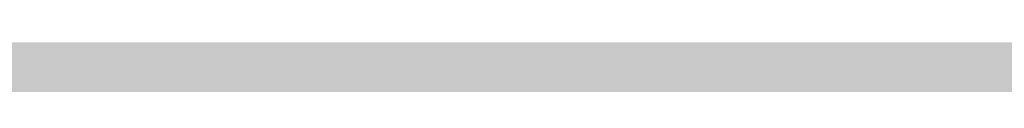
# Model space of a CAD drawing. Units: feet. Extents: x 3168 to 4724, y 827 to 1477.
# Tile 151 of 256: x 3301.1638 to 3301.19778, y 1099.01485 to 1099.01628. Entities that reach past the tile are written whole.
import ezdxf

# ---------------------------------------------------------------- set-up
doc = ezdxf.new("R2010")
doc.units = ezdxf.units.FT
doc.layers.add('A-ELEV', color=7, linetype='Continuous', lineweight=35)
doc.layers.add('A-ELEV-PATT', color=8, linetype='Continuous', lineweight=13)

msp = doc.modelspace()

# ---------------------------------------------------------------- hatches: boundary and pattern name
at = {"layer": 'A-ELEV-PATT'}
h = msp.add_hatch(color=256, dxfattribs=at)
h.dxf.hatch_style = 1
edge = h.paths.add_edge_path()
edge.add_ellipse((3552.905762, 979.220141), major_axis=(36.744924, 0), ratio=0.484848485, start_angle=0, end_angle=360)
edge = h.paths.add_edge_path()
edge.add_ellipse((3559.891637, 929.252282), major_axis=(36.744924, 0), ratio=0.484848485, start_angle=0, end_angle=360)
edge = h.paths.add_edge_path()
edge.add_line((3299.31681, 1198.606081), (3479.916714, 1198.606081))
edge.add_line((3479.916714, 1198.606081), (3479.916714, 1209.86857))
edge.add_spline(control_points=[(3479.916714, 1209.86857), (3464.301157, 1209.86857), (3448.685601, 1209.86857), (3410.949139, 1209.86857), (3388.828234, 1209.86857), (3355.646876, 1209.86857), (3344.586423, 1209.86857), (3327.995745, 1209.86857), (3322.465518, 1209.86857), (3314.170179, 1209.86857), (3311.405066, 1209.86857), (3307.257396, 1209.86857), (3305.874839, 1209.86857), (3303.801005, 1209.86857), (3303.109726, 1209.86857), (3302.072809, 1209.86857), (3301.72717, 1209.86857), (3301.208711, 1209.86857), (3301.035891, 1209.86857), (3300.776662, 1209.86857), (3300.690252, 1209.86857), (3300.560638, 1209.86857), (3300.517433, 1209.86857), (3300.452625, 1209.86857), (3300.431023, 1209.86857), (3300.398619, 1209.86857), (3300.387818, 1209.86857), (3300.366216, 1209.86857), (3300.345676, 1209.86857), (3300.345548, 1209.86857), (3300.345505, 1209.86857), (3300.343304, 1209.86857), (3300.341146, 1209.868571), (3300.337909, 1209.868571), (3300.33683, 1209.868572), (3300.333942, 1209.868573), (3300.332133, 1209.868574), (3300.325515, 1209.868577), (3300.320706, 1209.868581), (3300.310925, 1209.868592), (3300.305952, 1209.868598), (3300.290511, 1209.868623), (3300.280045, 1209.868646), (3300.232425, 1209.868777), (3300.195298, 1209.868954), (3299.951068, 1209.870608), (3299.744824, 1209.874326), (3299.436827, 1209.883257), (3299.334389, 1209.886792), (3299.181079, 1209.89292), (3299.130033, 1209.895099), (3298.652217, 1209.916801), (3298.22946, 1209.945718), (3297.601631, 1210.002367), (3297.393404, 1210.023464), (3297.082652, 1210.058309), (3296.979332, 1210.070458), (3296.292954, 1210.154861), (3295.718148, 1210.243356), (3294.868717, 1210.39885), (3294.5877, 1210.454478), (3294.169341, 1210.543349), (3294.030415, 1210.573878), (3291.707149, 1211.1012), (3289.65359, 1211.813435), (3285.776259, 1213.563988), (3283.95141, 1214.603478), (3280.512159, 1216.98008), (3278.897241, 1218.317592), (3276.379914, 1220.829489), (3275.416042, 1221.917738), (3274.039342, 1223.7077), (3273.581043, 1224.349535), (3273.143228, 1225.016316)], knot_values=[39.119033, 39.119033, 39.119033, 39.119033, 39.286353, 39.286353, 39.523379, 39.523379, 39.641892, 39.641892, 39.701148, 39.701148, 39.730777, 39.730777, 39.745591, 39.745591, 39.752998, 39.752998, 39.756701, 39.756701, 39.758553, 39.758553, 39.759479, 39.759479, 39.759942, 39.759942, 39.760173, 39.760173, 39.760289, 39.760289, 39.760405, 39.760405, 39.760463, 39.760463, 39.763389, 39.763389, 39.764851, 39.764851, 39.767304, 39.767304, 39.773825, 39.773825, 39.78057, 39.78057, 39.79477, 39.79477, 39.845194, 39.845194, 40.126715, 40.126715, 40.267476, 40.267476, 40.337856, 40.337856, 40.927023, 40.927023, 41.221606, 41.221606, 41.368898, 41.368898, 42.202622, 42.202622, 42.619485, 42.619485, 42.827916, 42.827916, 46.118323, 46.118323, 49.408731, 49.408731, 52.699139, 52.699139, 54.927489, 54.927489, 56.104228, 56.104228, 56.104228, 56.104228], weights=[1, 1, 1, 1, 1, 1, 1, 1, 1, 1, 1, 1, 1, 1, 1, 1, 1, 1, 1, 1, 1, 1, 1, 1, 1, 1, 1, 1, 1, 1, 1, 1, 1, 1, 1, 1, 1, 1, 1, 1, 1, 1, 1, 1, 1, 1, 1, 1, 1, 1, 1, 1, 1, 1, 1, 1, 1, 1, 1, 1, 1, 1, 1, 1, 1, 1, 1, 1, 1, 1, 1, 1, 1, 1], degree=3, periodic=0)
edge.add_line((3273.143228, 1225.016316), (3273.143228, 1099.016316))
edge.add_line((3273.143228, 1099.016316), (3299.31681, 1099.016316))
edge.add_line((3299.31681, 1099.016316), (3299.31681, 1198.606081))
edge = h.paths.add_edge_path()
edge.add_line((3304.758443, 1324.15806), (3479.916714, 1324.15806))
edge.add_line((3479.916714, 1324.15806), (3479.916714, 1335.714618))
edge.add_line((3479.916714, 1335.714618), (3269.161628, 1335.714618))
edge.add_spline(control_points=[(3269.161628, 1335.714618), (3264.024231, 1335.714618), (3258.364118, 1328.958189), (3259.264311, 1323.900274)], knot_values=[0, 0, 0, 0, 15.412191, 15.412191, 15.412191, 15.412191], degree=3, periodic=0)
edge.add_line((3259.264311, 1323.900274), (3265.516849, 1288.769135))
edge.add_line((3265.516849, 1288.769135), (3275.265103, 1261.545626))
edge.add_line((3275.265103, 1261.545626), (3304.758443, 1261.545626))
edge.add_line((3304.758443, 1261.545626), (3304.758443, 1324.15806))
h = msp.add_hatch(color=256, dxfattribs=at)
h.dxf.hatch_style = 1
h.paths.add_polyline_path([(3384.525247, 1099.016316), (3335.029168, 1099.016316), (3299.31681, 1099.016316), (3273.143228, 1099.016316), (3217.565364, 1099.016316), (3168.069285, 827.11626), (3335.029168, 827.11626)])

# ---------------------------------------------------------------- linework, layer by layer
at = {"layer": 'A-ELEV'}
msp.add_open_spline([(3808.5202, 1099.016316), (3808.5202, 1141.413235), (3808.5202, 1183.810154), (3808.5202, 1226.635324), (3808.5202, 1227.063576), (3808.5202, 1227.491828), (3811.491871, 1248.994673), (3814.463542, 1270.497518), (3817.46523, 1292.217564), (3817.495247, 1292.434764), (3817.525264, 1292.651964), (3817.572801, 1310.106748), (3817.620339, 1327.561532), (3817.667877, 1345.016316), (3817.667877, 1345.457962), (3817.667877, 1345.899608), (3817.667877, 1346.456047), (3817.667877, 1346.57084), (3817.667877, 1346.752887), (3817.667877, 1346.820142), (3817.667877, 1346.93487), (3817.667877, 1346.982345), (3817.667877, 1347.038587), (3817.667877, 1347.047356), (3817.667877, 1347.073661), (3817.667877, 1347.059303), (3817.667877, 1347.061545), (3817.667876, 1347.062667), (3817.667875, 1347.066031), (3817.667874, 1347.068274), (3817.66787, 1347.075001), (3817.667866, 1347.079486), (3817.667849, 1347.092937), (3817.667833, 1347.101902), (3817.667766, 1347.12879), (3817.667699, 1347.146705), (3817.667432, 1347.200421), (3817.667165, 1347.236192), (3817.6661, 1347.343385), (3817.665038, 1347.414686), (3817.660812, 1347.628095), (3817.656608, 1347.769708), (3817.63997, 1348.192487), (3817.623509, 1348.471586), (3817.559094, 1349.300067), (3817.496121, 1349.840588), (3817.255432, 1351.424156), (3817.026318, 1352.428785), (3816.306871, 1354.888914), (3815.743745, 1356.268727), (3814.463959, 1358.81921), (3813.746413, 1359.990968), (3812.195838, 1362.172343), (3811.362245, 1363.182124), (3809.588836, 1365.069009), (3808.648816, 1365.946105), (3806.654262, 1367.579616), (3805.599702, 1368.336154), (3803.352891, 1369.722327), (3802.160535, 1370.352386), (3799.600813, 1371.453586), (3798.232688, 1371.925481), (3795.280084, 1372.634624), (3793.693148, 1372.872068), (3791.869441, 1372.92648), (3791.740861, 1372.92922), (3791.353371, 1372.934101), (3791.092707, 1372.932901), (3790.304116, 1372.915068), (3789.769543, 1372.884195), (3789.20919, 1372.830236), (3789.190622, 1372.828424), (3789.134892, 1372.822912), (3789.097705, 1372.819137), (3789.048445, 1372.814008), (3789.0364, 1372.812743), (3789.000256, 1372.808918), (3788.976147, 1372.806325), (3788.949405, 1372.803404), (3788.946786, 1372.803118), (3788.942567, 1372.802655), (3788.940967, 1372.80248), (3788.938572, 1372.802217), (3788.937777, 1372.802129), (3788.935391, 1372.801867), (3788.867535, 1372.794402), (3788.756866, 1372.782228), (3788.701532, 1372.776141), (3788.53553, 1372.75788), (3788.424861, 1372.745707), (3788.092856, 1372.709185), (3787.871519, 1372.684837), (3787.207509, 1372.611793), (3786.764835, 1372.563097), (3785.436814, 1372.417009), (3784.551467, 1372.319617), (3781.895425, 1372.027442), (3780.12473, 1371.832658), (3774.812646, 1371.248307), (3771.271256, 1370.858739), (3760.647088, 1369.690037), (3753.56431, 1368.910902), (3732.315973, 1366.573498), (3718.150416, 1365.015228), (3694.006758, 1362.359326), (3684.028657, 1361.261694), (3674.050557, 1360.164062), (3664.600662, 1360.164062), (3655.150767, 1360.164062), (3626.801081, 1360.164062), (3607.901291, 1360.164062), (3551.20192, 1360.164062), (3513.40234, 1360.164062), (3467.725182, 1360.164062), (3459.847604, 1360.164062), (3436.214873, 1360.164062), (3420.459718, 1360.164062), (3373.194255, 1360.164062), (3341.683946, 1360.164062), (3302.848162, 1360.164062), (3295.522686, 1360.164062), (3286.038292, 1360.164062), (3283.879372, 1360.164062), (3277.402613, 1360.164062), (3273.084773, 1360.164062), (3267.732851, 1360.164062), (3266.698768, 1360.164062), (3263.59652, 1360.164062), (3261.528355, 1360.164062), (3259.236943, 1360.164062), (3259.013697, 1360.164062), (3258.343958, 1360.164062), (3257.897466, 1360.164062), (3257.430998, 1360.164062), (3257.411022, 1360.164062), (3257.370573, 1360.164062), (3257.37547, 1360.164062), (3257.374598, 1360.164062), (3257.373937, 1360.164062), (3257.371956, 1360.164062), (3257.370635, 1360.164061), (3257.366673, 1360.16406), (3257.364032, 1360.164059), (3257.356109, 1360.164053), (3257.350828, 1360.164047), (3257.334987, 1360.164023), (3257.32443, 1360.163998), (3257.292769, 1360.163899), (3257.271676, 1360.163799), (3257.208439, 1360.163398), (3257.166337, 1360.162995), (3257.040206, 1360.161388), (3256.956349, 1360.159783), (3256.705504, 1360.153393), (3256.53924, 1360.147036), (3256.04357, 1360.121916), (3255.717296, 1360.097102), (3254.752446, 1360.000481), (3254.127968, 1359.906513), (3252.180067, 1359.525332), (3250.941574, 1359.143991), (3248.670175, 1358.24329), (3247.635739, 1357.723834), (3245.732632, 1356.603471), (3244.863388, 1356.00206), (3243.253108, 1354.742865), (3242.511972, 1354.084731), (3240.751052, 1352.344781), (3239.800961, 1351.229574), (3238.087769, 1348.87244), (3237.324685, 1347.630355), (3235.98251, 1344.971632), (3235.402205, 1343.554907), (3234.591081, 1340.815458), (3234.310882, 1339.54355), (3233.97649, 1336.802561), (3233.922113, 1335.330877), (3234.148916, 1332.591269), (3234.349529, 1331.367201), (3234.719893, 1329.999367), (3234.752423, 1329.883362), (3234.853619, 1329.534797), (3234.925892, 1329.301685), (3235.024836, 1329.002552), (3235.046924, 1328.936928), (3235.077639, 1328.847239), (3235.085924, 1328.823198), (3235.110939, 1328.751064), (3235.127828, 1328.702962), (3235.147992, 1328.646242), (3235.151059, 1328.637632), (3235.156096, 1328.623526), (3235.158061, 1328.61803), (3235.160209, 1328.61203), (3235.165612, 1328.596943), (3235.180099, 1328.556486), (3235.190263, 1328.528101), (3235.220756, 1328.442946), (3235.241084, 1328.386176), (3235.302069, 1328.215865), (3235.342726, 1328.102325), (3235.464696, 1327.761704), (3235.54601, 1327.534623), (3235.78995, 1326.853381), (3235.952577, 1326.39922), (3236.440459, 1325.036736), (3236.765713, 1324.128414), (3237.741475, 1321.403446), (3238.391983, 1319.586801), (3240.343508, 1314.136866), (3241.644525, 1310.503576), (3245.547574, 1299.603706), (3248.149607, 1292.337126), (3255.955706, 1270.537385), (3261.159772, 1256.004225), (3267.387618, 1238.612001), (3268.411397, 1235.752937), (3269.510378, 1232.683864), (3269.585579, 1232.473854), (3269.706612, 1232.135851), (3269.752444, 1232.007857), (3269.827329, 1231.79873), (3269.856382, 1231.717595), (3269.906325, 1231.578122), (3269.927215, 1231.519782), (3269.972468, 1231.393406), (3269.996831, 1231.325368), (3270.026503, 1231.242506), (3270.031811, 1231.227681), (3270.040282, 1231.204024), (3270.039224, 1231.206979), (3270.039359, 1231.206601), (3270.039427, 1231.206412), (3270.03963, 1231.205846), (3270.039765, 1231.205468), (3270.040171, 1231.204335), (3270.040442, 1231.203579), (3270.041254, 1231.201313), (3270.041796, 1231.199802), (3270.04342, 1231.195269), (3270.044504, 1231.192248), (3270.047756, 1231.183185), (3270.049926, 1231.177145), (3270.056442, 1231.159028), (3270.060793, 1231.146957), (3270.073867, 1231.110761), (3270.082613, 1231.086656), (3270.108936, 1231.014413), (3270.1266, 1230.96635), (3270.179934, 1230.822457), (3270.215947, 1230.726923), (3270.325323, 1230.441508), (3270.400026, 1230.252811), (3270.629249, 1229.691444), (3270.788883, 1229.323501), (3271.286488, 1228.238319), (3271.6431, 1227.539755), (3272.775859, 1225.515277), (3273.614169, 1224.260502), (3275.416042, 1221.917738), (3276.379914, 1220.829489), (3278.897241, 1218.317592), (3280.512159, 1216.98008), (3283.95141, 1214.603478), (3285.776259, 1213.563988), (3289.65359, 1211.813435), (3291.707149, 1211.1012), (3294.030415, 1210.573878), (3294.169341, 1210.543349), (3294.5877, 1210.454478), (3294.868717, 1210.39885), (3295.718148, 1210.243356), (3296.292954, 1210.154861), (3296.979332, 1210.070458), (3297.082652, 1210.058309), (3297.393404, 1210.023464), (3297.601631, 1210.002367), (3298.22946, 1209.945718), (3298.652217, 1209.916801), (3299.130033, 1209.895099), (3299.181079, 1209.89292), (3299.334389, 1209.886792), (3299.436827, 1209.883257), (3299.744824, 1209.874326), (3299.951068, 1209.870608), (3300.195298, 1209.868954), (3300.232425, 1209.868777), (3300.280045, 1209.868646), (3300.290511, 1209.868623), (3300.305952, 1209.868598), (3300.310925, 1209.868592), (3300.320706, 1209.868581), (3300.325515, 1209.868577), (3300.332133, 1209.868574), (3300.333942, 1209.868573), (3300.33683, 1209.868572), (3300.337909, 1209.868571), (3300.341146, 1209.868571), (3300.343304, 1209.86857), (3300.345505, 1209.86857), (3300.345548, 1209.86857), (3300.345676, 1209.86857), (3300.366216, 1209.86857), (3300.387818, 1209.86857), (3300.398619, 1209.86857), (3300.431023, 1209.86857), (3300.452625, 1209.86857), (3300.517433, 1209.86857), (3300.560638, 1209.86857), (3300.690252, 1209.86857), (3300.776662, 1209.86857), (3301.035891, 1209.86857), (3301.208711, 1209.86857), (3301.72717, 1209.86857), (3302.072809, 1209.86857), (3303.109726, 1209.86857), (3303.801005, 1209.86857), (3305.874839, 1209.86857), (3307.257396, 1209.86857), (3311.405066, 1209.86857), (3314.170179, 1209.86857), (3322.465518, 1209.86857), (3327.995745, 1209.86857), (3344.586423, 1209.86857), (3355.646876, 1209.86857), (3388.828234, 1209.86857), (3410.949139, 1209.86857), (3477.311855, 1209.86857), (3521.553665, 1209.86857), (3566.836184, 1209.86857), (3567.876892, 1209.86857), (3570.999017, 1209.86857), (3573.080433, 1209.86857), (3575.781396, 1209.86857), (3576.400943, 1209.86857), (3577.295821, 1209.86857), (3577.571152, 1209.86857), (3578.397146, 1209.86857), (3578.947808, 1209.86857), (3579.756491, 1209.86857), (3580.014511, 1209.86857), (3580.342737, 1209.86857), (3580.326865, 1209.86857), (3580.32717, 1209.86857), (3580.327323, 1209.86857), (3580.327781, 1209.86857), (3580.328086, 1209.86857), (3580.329002, 1209.86857), (3580.329613, 1209.86857), (3580.331445, 1209.86857), (3580.332667, 1209.86857), (3580.336332, 1209.868569), (3580.338775, 1209.868567), (3580.346107, 1209.868563), (3580.350995, 1209.868558), (3580.365663, 1209.86854), (3580.375445, 1209.868522), (3580.404801, 1209.868449), (3580.424386, 1209.868376), (3580.483183, 1209.868085), (3580.522437, 1209.867793), (3580.640361, 1209.866624), (3580.719195, 1209.865454), (3580.956315, 1209.860766), (3581.115222, 1209.85607), (3581.594164, 1209.83723), (3581.916419, 1209.818331), (3582.889947, 1209.742428), (3583.547986, 1209.666169), (3585.531827, 1209.360617), (3586.867216, 1209.053886), (3589.471545, 1208.252472), (3590.740241, 1207.757852), (3591.995451, 1207.158802), (3592.057809, 1207.12874), (3592.244242, 1207.037954), (3592.367676, 1206.976632), (3592.73528, 1206.790359), (3592.976752, 1206.663101), (3593.244539, 1206.516441), (3593.274731, 1206.499825), (3593.365115, 1206.449839), (3593.425113, 1206.416333), (3593.604314, 1206.315285), (3593.722725, 1206.247211), (3593.857212, 1206.168398), (3593.874362, 1206.158319), (3593.925741, 1206.128041), (3593.959899, 1206.107798), (3594.062086, 1206.046899), (3594.129827, 1206.006074), (3594.208436, 1205.958171), (3594.219683, 1205.951304), (3594.253391, 1205.930686), (3594.275819, 1205.916917), (3594.342972, 1205.875536), (3594.387563, 1205.847853), (3594.433616, 1205.81905), (3594.435256, 1205.818024), (3594.440175, 1205.814946), (3594.443453, 1205.812894), (3594.447123, 1205.810594), (3594.447516, 1205.810348), (3594.448695, 1205.80961), (3594.449481, 1205.809117), (3594.450366, 1205.808562), (3594.450466, 1205.8085), (3594.4506, 1205.808415), (3594.467399, 1205.797887), (3594.493269, 1205.781674), (3594.506204, 1205.773568), (3594.545008, 1205.749248), (3594.570878, 1205.733035), (3594.648487, 1205.684396), (3594.700226, 1205.651969), (3594.855444, 1205.554691), (3594.958922, 1205.489839), (3595.269357, 1205.295282), (3595.476314, 1205.165577), (3596.097185, 1204.776463), (3596.511099, 1204.517054), (3597.752841, 1203.738826), (3598.580669, 1203.220007), (3601.064152, 1201.663551), (3602.719807, 1200.625914), (3607.686774, 1197.513002), (3610.998085, 1195.437727), (3620.932018, 1189.211903), (3627.55464, 1185.061354), (3647.422507, 1172.609707), (3660.667751, 1164.308608), (3700.403484, 1139.405313), (3726.893973, 1122.803116), (3757.205715, 1103.806052), (3761.02697, 1101.411184), (3764.848224, 1099.016316), (3745.328271, 1099.016316), (3725.808319, 1099.016316), (3706.288366, 1099.016316), (3706.288366, 1108.453237), (3706.288366, 1117.890158), (3706.288366, 1127.327079), (3710.750754, 1127.327079), (3715.213143, 1127.327079), (3719.675531, 1127.327079)], degree=3, knots=[0, 0, 0, 0, 0.982037, 0.982037, 0.991957, 0.991957, 0.991957, 1.966522, 1.966522, 1.976367, 1.976367, 1.976367, 2.976367, 2.976367, 2.976367, 3.00169, 3.00169, 3.008272, 3.008272, 3.012129, 3.012129, 3.014851, 3.014851, 3.015353, 3.015353, 3.016359, 3.016359, 3.017365, 3.017365, 3.019376, 3.019376, 3.023398, 3.023398, 3.031442, 3.031442, 3.047531, 3.047531, 3.079708, 3.079708, 3.144063, 3.144063, 3.272772, 3.272772, 3.53019, 3.53019, 4.045026, 4.045026, 5.074698, 5.074698, 6.700878, 6.700878, 8.327058, 8.327058, 9.953238, 9.953238, 11.579418, 11.579418, 13.205598, 13.205598, 14.831778, 14.831778, 16.457958, 16.457958, 18.084138, 18.084138, 18.206872, 18.206872, 18.45234, 18.45234, 18.943275, 18.943275, 18.960093, 18.960093, 18.993729, 18.993729, 19.00461, 19.00461, 19.026374, 19.026374, 19.028737, 19.028737, 19.03018, 19.03018, 19.030897, 19.030897, 19.032332, 19.032332, 19.033766, 19.033766, 19.036636, 19.036636, 19.042374, 19.042374, 19.053851, 19.053851, 19.076805, 19.076805, 19.122714, 19.122714, 19.21453, 19.21453, 19.398163, 19.398163, 19.765429, 19.765429, 20.024128, 20.024128, 20.024128, 20.092031, 20.092031, 20.227836, 20.227836, 20.499446, 20.499446, 20.556051, 20.556051, 20.66926, 20.66926, 20.895678, 20.895678, 20.948316, 20.948316, 20.963829, 20.963829, 20.994855, 20.994855, 21.002285, 21.002285, 21.017146, 21.017146, 21.01875, 21.01875, 21.021959, 21.021959, 21.022102, 21.022102, 21.022249, 21.022249, 21.022708, 21.022708, 21.023627, 21.023627, 21.025464, 21.025464, 21.029138, 21.029138, 21.036486, 21.036486, 21.051183, 21.051183, 21.080575, 21.080575, 21.139361, 21.139361, 21.256932, 21.256932, 21.492073, 21.492073, 21.962356, 21.962356, 23.01002, 23.01002, 24.057684, 24.057684, 25.105348, 25.105348, 26.153011, 26.153011, 27.776787, 27.776787, 29.400562, 29.400562, 31.024337, 31.024337, 32.278801, 32.278801, 33.533265, 33.533265, 34.467568, 34.467568, 34.553971, 34.553971, 34.726776, 34.726776, 34.775309, 34.775309, 34.793079, 34.793079, 34.82862, 34.82862, 34.834979, 34.834979, 34.839039, 34.839039, 34.839411, 34.839411, 34.840285, 34.840285, 34.842034, 34.842034, 34.845531, 34.845531, 34.852525, 34.852525, 34.866512, 34.866512, 34.894488, 34.894488, 34.950439, 34.950439, 35.062342, 35.062342, 35.286147, 35.286147, 35.733758, 35.733758, 35.821815, 35.821815, 35.828283, 35.828283, 35.832225, 35.832225, 35.834724, 35.834724, 35.836521, 35.836521, 35.838617, 35.838617, 35.839073, 35.839073, 35.839345, 35.839345, 35.839617, 35.839617, 35.840161, 35.840161, 35.841249, 35.841249, 35.843425, 35.843425, 35.847778, 35.847778, 35.856482, 35.856482, 35.873891, 35.873891, 35.908709, 35.908709, 35.978345, 35.978345, 36.117617, 36.117617, 36.396161, 36.396161, 36.953248, 36.953248, 38.067423, 38.067423, 40.295772, 40.295772, 42.524122, 42.524122, 45.81453, 45.81453, 49.104937, 49.104937, 52.395345, 52.395345, 52.603776, 52.603776, 53.020639, 53.020639, 53.854363, 53.854363, 54.001655, 54.001655, 54.296238, 54.296238, 54.885405, 54.885405, 54.955785, 54.955785, 55.096546, 55.096546, 55.378067, 55.378067, 55.42849, 55.42849, 55.442691, 55.442691, 55.449436, 55.449436, 55.455957, 55.455957, 55.458409, 55.458409, 55.459872, 55.459872, 55.462798, 55.462798, 55.462856, 55.462856, 55.462972, 55.462972, 55.463088, 55.463088, 55.463319, 55.463319, 55.463782, 55.463782, 55.464708, 55.464708, 55.46656, 55.46656, 55.470263, 55.470263, 55.47767, 55.47767, 55.492484, 55.492484, 55.522112, 55.522112, 55.581369, 55.581369, 55.699882, 55.699882, 55.936907, 55.936907, 56.410959, 56.410959, 56.42211, 56.42211, 56.444413, 56.444413, 56.451051, 56.451051, 56.454001, 56.454001, 56.459901, 56.459901, 56.462666, 56.462666, 56.463418, 56.463418, 56.464171, 56.464171, 56.465675, 56.465675, 56.468684, 56.468684, 56.474702, 56.474702, 56.486738, 56.486738, 56.51081, 56.51081, 56.558955, 56.558955, 56.655243, 56.655243, 56.847821, 56.847821, 57.232975, 57.232975, 58.003284, 58.003284, 59.543901, 59.543901, 62.625137, 62.625137, 68.787607, 68.787607, 74.950078, 74.950078, 75.27336, 75.27336, 75.919923, 75.919923, 77.213051, 77.213051, 77.377769, 77.377769, 77.707206, 77.707206, 78.366079, 78.366079, 78.462532, 78.462532, 78.655436, 78.655436, 79.041245, 79.041245, 79.105735, 79.105735, 79.234714, 79.234714, 79.492672, 79.492672, 79.502197, 79.502197, 79.521249, 79.521249, 79.523534, 79.523534, 79.528103, 79.528103, 79.528682, 79.528682, 79.528885, 79.528885, 79.529089, 79.529089, 79.529495, 79.529495, 79.530308, 79.530308, 79.531935, 79.531935, 79.535187, 79.535187, 79.541693, 79.541693, 79.554704, 79.554704, 79.580725, 79.580725, 79.632769, 79.632769, 79.736856, 79.736856, 79.94503, 79.94503, 80.361377, 80.361377, 80.421435, 80.421435, 80.421435, 81.421435, 81.421435, 81.421435, 82.421435, 82.421435, 82.421435, 83.421435, 83.421435, 83.421435, 83.421435], dxfattribs=at)

doc.saveas('drawing.dxf')
